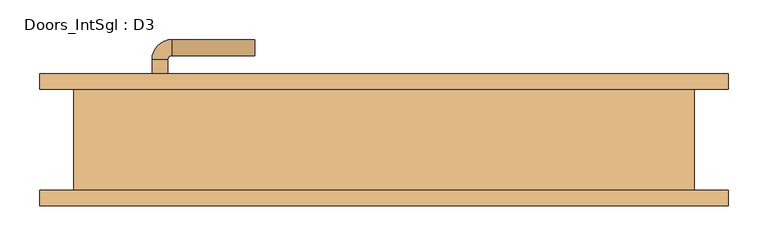
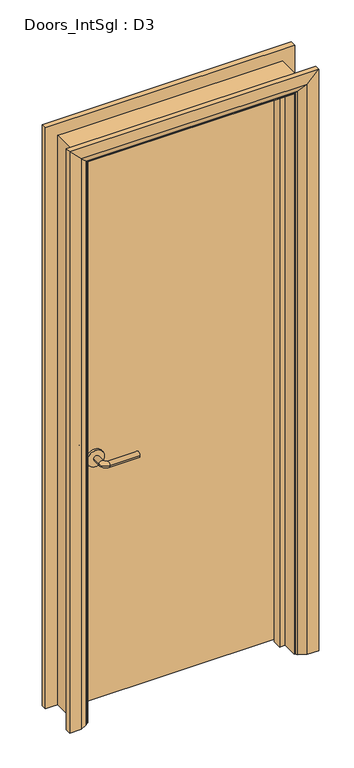
"""IFC4 building model written with IfcOpenShell, lengths in millimetres: door geometry, Doors_IntSgl : D3."""

from ifc_helpers import new_model, si_unit, point, frame, frame_2d, origin, place, context, project, spatial, polyline, circle_curve, ellipse_curve, trimmed, segment, composite_curve, outline, extrude, faceted_brep, source, transform, mapped, element, save
from ifc_brep_helpers import plane_surface, cylinder_surface, revolved_surface, advanced_brep


def doors_intsgl_d3_a25f8c6e(model_context):
    return source(origin(), model_context, "Body", "SolidModel", [
        advanced_brep(
        [(-293.05, 17.5, 900.0), (-273.05, 17.5, 900.0), (-273.05, -12.5, 900.0), (-293.05, -12.5, 900.0), (-268.05, -17.5, 900.0), (-268.05, -37.5, 900.0), (-163.05, -37.5, 900.0), (-163.05, -17.5, 900.0)],
        [
            (0, 1, circle_curve(frame((-283.05, 17.5, 900.0), z_axis=(0.0, 1.0, 0.0), x_axis=(1.0, 0.0, 0.0)), 10.0)),
            (1, 0, circle_curve(frame((-283.05, 17.5, 900.0), z_axis=(0.0, 1.0, 0.0), x_axis=(1.0, 0.0, 0.0)), 10.0)),
            (1, 2),
            (2, 3, circle_curve(frame((-283.05, -12.5, 900.0), z_axis=(0.0, 1.0, 0.0), x_axis=(1.0, 0.0, 0.0)), 10.0)),
            (3, 0),
            (3, 2, circle_curve(frame((-283.05, -12.5, 900.0), z_axis=(0.0, 1.0, 0.0), x_axis=(1.0, 0.0, 0.0)), 10.0)),
            (4, 5, circle_curve(frame((-268.05, -27.5, 900.0), z_axis=(-1.0, 0.0, 0.0), x_axis=(0.0, 1.0, 0.0)), 10.0)),
            (5, 3, circle_curve(frame((-268.05, -12.5, 900.0), z_axis=(0.0, 0.0, -1.0), x_axis=(-1.0, 0.0, 0.0)), 25.0)),
            (2, 4, circle_curve(frame((-268.05, -12.5, 900.0), z_axis=(0.0, 0.0, 1.0), x_axis=(-1.0, 0.0, 0.0)), 5.0)),
            (5, 4, circle_curve(frame((-268.05, -27.5, 900.0), z_axis=(-1.0, 0.0, 0.0), x_axis=(0.0, 1.0, 0.0)), 10.0)),
            (6, 7, circle_curve(frame((-163.05, -27.5, 900.0), z_axis=(1.0, 0.0, 0.0), x_axis=(0.0, 1.0, 0.0)), 10.0)),
            (7, 6, circle_curve(frame((-163.05, -27.5, 900.0), z_axis=(1.0, 0.0, 0.0), x_axis=(0.0, 1.0, 0.0)), 10.0)),
            (4, 7),
            (6, 5),
        ],
        [
            plane_surface(frame((-283.05, 17.5, 900.0), z_axis=(0.0, 1.0, 0.0), x_axis=(0.0, 0.0, 1.0))),
            cylinder_surface(frame((-283.05, 17.5, 900.0), z_axis=(0.0, 1.0, 0.0), x_axis=(1.0, 0.0, 0.0)), 10.0),
            revolved_surface(trimmed(ellipse_curve(frame((-283.05, -12.5, 900.0), z_axis=(0.0, -1.0, 0.0), x_axis=(1.0, 0.0, 0.0)), 10.0, 10.0), [point((-293.05, -12.5, 900.0))], [point((-273.05, -12.5, 900.0))], True, "CARTESIAN"), (-268.05, -12.5, 900.0), (0.0, 0.0, -1.0)),
            revolved_surface(trimmed(ellipse_curve(frame((-283.05, -12.5, 900.0), z_axis=(0.0, -1.0, 0.0), x_axis=(1.0, 0.0, 0.0)), 10.0, 10.0), [point((-273.05, -12.5, 900.0))], [point((-293.05, -12.5, 900.0))], True, "CARTESIAN"), (-268.05, -12.5, 900.0), (0.0, 0.0, -1.0)),
            plane_surface(frame((-163.05, -27.5, 900.0), z_axis=(1.0, 0.0, 0.0), x_axis=(0.0, 0.0, 1.0))),
            cylinder_surface(frame((-268.05, -27.5, 900.0), z_axis=(-1.0, 0.0, 0.0), x_axis=(0.0, 1.0, 0.0)), 10.0),
        ],
        [
            (0, [[1, 2]]),
            (1, [[3, 4, 5, -2]]),
            (1, [[-5, 6, -3, -1]]),
            (2, [[7, 8, -4, 9]]),
            (3, [[10, -9, -6, -8]]),
            (4, [[11, 12]]),
            (5, [[13, -11, 14, -7]]),
            (5, [[-14, -12, -13, -10]]),
        ],
    ),
        extrude(outline(composite_curve([segment(trimmed(circle_curve(frame_2d((900.0, -285.55)), 30.0), [point((900.0, -315.55))], [point((900.0, -255.55))], False, "CARTESIAN"), True, "CONTINUOUS"), segment(trimmed(circle_curve(frame_2d((900.0, -285.55)), 30.0), [point((900.0, -255.55))], [point((900.0, -315.55))], False, "CARTESIAN"), True, "CONTINUOUS")], self_intersect=False)), frame((0.0, 17.5, 0.0), z_axis=(0.0, 1.0, 0.0), x_axis=(0.0, 0.0, 1.0)), (0.0, 0.0, 1.0), 8.0),
        advanced_brep(
        [(-293.05, 71.5, 900.0), (-273.05, 71.5, 900.0), (-293.05, 101.5, 900.0), (-273.05, 101.5, 900.0), (-268.05, 106.5, 900.0), (-268.05, 126.5, 900.0), (-163.05, 126.5, 900.0), (-163.05, 106.5, 900.0)],
        [
            (0, 1, circle_curve(frame((-283.05, 71.5, 900.0), z_axis=(0.0, -1.0, 0.0), x_axis=(1.0, 0.0, 0.0)), 10.0)),
            (1, 0, circle_curve(frame((-283.05, 71.5, 900.0), z_axis=(0.0, -1.0, 0.0), x_axis=(1.0, 0.0, 0.0)), 10.0)),
            (0, 2),
            (2, 3, circle_curve(frame((-283.05, 101.5, 900.0), z_axis=(0.0, -1.0, 0.0), x_axis=(1.0, 0.0, 0.0)), 10.0)),
            (3, 1),
            (3, 2, circle_curve(frame((-283.05, 101.5, 900.0), z_axis=(0.0, -1.0, 0.0), x_axis=(1.0, 0.0, 0.0)), 10.0)),
            (4, 3, circle_curve(frame((-268.05, 101.5, 900.0), z_axis=(0.0, 0.0, 1.0), x_axis=(-1.0, 0.0, 0.0)), 5.0)),
            (2, 5, circle_curve(frame((-268.05, 101.5, 900.0), z_axis=(0.0, 0.0, -1.0), x_axis=(-1.0, 0.0, 0.0)), 25.0)),
            (5, 4, circle_curve(frame((-268.05, 116.5, 900.0), z_axis=(-1.0, 0.0, 0.0), x_axis=(0.0, -1.0, 0.0)), 10.0)),
            (4, 5, circle_curve(frame((-268.05, 116.5, 900.0), z_axis=(-1.0, 0.0, 0.0), x_axis=(0.0, -1.0, 0.0)), 10.0)),
            (6, 7, circle_curve(frame((-163.05, 116.5, 900.0), z_axis=(1.0, 0.0, 0.0), x_axis=(0.0, -1.0, 0.0)), 10.0)),
            (7, 6, circle_curve(frame((-163.05, 116.5, 900.0), z_axis=(1.0, 0.0, 0.0), x_axis=(0.0, -1.0, 0.0)), 10.0)),
            (5, 6),
            (7, 4),
        ],
        [
            plane_surface(frame((-283.05, 71.5, 900.0), z_axis=(0.0, -1.0, 0.0), x_axis=(0.0, 0.0, 1.0))),
            cylinder_surface(frame((-283.05, 71.5, 900.0), z_axis=(0.0, -1.0, 0.0), x_axis=(1.0, 0.0, 0.0)), 10.0),
            revolved_surface(trimmed(ellipse_curve(frame((-283.05, 101.5, 900.0), z_axis=(0.0, -1.0, 0.0), x_axis=(1.0, 0.0, 0.0)), 10.0, 10.0), [point((-293.05, 101.5, 900.0))], [point((-273.05, 101.5, 900.0))], True, "CARTESIAN"), (-268.05, 101.5, 900.0), (0.0, 0.0, -1.0)),
            revolved_surface(trimmed(ellipse_curve(frame((-283.05, 101.5, 900.0), z_axis=(0.0, -1.0, 0.0), x_axis=(1.0, 0.0, 0.0)), 10.0, 10.0), [point((-273.05, 101.5, 900.0))], [point((-293.05, 101.5, 900.0))], True, "CARTESIAN"), (-268.05, 101.5, 900.0), (0.0, 0.0, -1.0)),
            plane_surface(frame((-163.05, 116.5, 900.0), z_axis=(1.0, 0.0, 0.0), x_axis=(0.0, 0.0, 1.0))),
            cylinder_surface(frame((-268.05, 116.5, 900.0), z_axis=(-1.0, 0.0, 0.0), x_axis=(0.0, -1.0, 0.0)), 10.0),
        ],
        [
            (0, [[1, 2]]),
            (1, [[-1, 3, 4, 5]]),
            (1, [[-2, -5, 6, -3]]),
            (2, [[7, -4, 8, 9]]),
            (3, [[-8, -6, -7, 10]]),
            (4, [[11, 12]]),
            (5, [[-9, 13, -12, 14]]),
            (5, [[-10, -14, -11, -13]]),
        ],
    ),
        extrude(outline(composite_curve([segment(trimmed(circle_curve(frame_2d((900.0, -285.55)), 30.0), [point((900.0, -315.55))], [point((900.0, -255.55))], False, "CARTESIAN"), True, "CONTINUOUS"), segment(trimmed(circle_curve(frame_2d((900.0, -285.55)), 30.0), [point((900.0, -255.55))], [point((900.0, -315.55))], False, "CARTESIAN"), True, "CONTINUOUS")], self_intersect=False)), frame((0.0, 63.5, 0.0), z_axis=(0.0, 1.0, 0.0), x_axis=(0.0, 0.0, 1.0)), (0.0, 0.0, 1.0), 8.0),
        extrude(outline(polyline([(358.05, 25.5), (-358.05, 25.5), (-358.05, 63.5), (358.05, 63.5), (358.05, 25.5)])), frame((0.0, 0.0, 8.0), z_axis=(0.0, 0.0, 1.0), x_axis=(1.0, 0.0, 0.0)), (0.0, 0.0, 1.0), 2060.0),
        advanced_brep(
        [(435.05, 83.5, 0.0), (435.05, 63.5, 0.0), (365.05, 63.5, 0.0), (369.05, 69.5, 0.0), (395.05, 83.5, 0.0), (435.05, 83.5, 2145.0), (435.05, 63.5, 2145.0), (-435.05, 63.5, 2145.0), (-435.05, 63.5, 0.0), (-365.05, 63.5, 0.0), (-365.05, 63.5, 2075.0), (365.05, 63.5, 2075.0), (369.05, 69.5, 2079.0), (395.05, 83.5, 2105.0), (-395.05, 83.5, 2105.0), (-395.05, 83.5, 0.0), (-435.05, 83.5, 0.0), (-435.05, 83.5, 2145.0), (-369.05, 69.5, 0.0), (-369.05, 69.5, 2079.0)],
        [
            (0, 1),
            (1, 2),
            (2, 3, circle_curve(frame((373.05, 62.5, 0.0), z_axis=(0.0, 0.0, -1.0), x_axis=(1.0, 0.0, 0.0)), 8.0622577)),
            (3, 4),
            (4, 0),
            (0, 5),
            (5, 6),
            (6, 1),
            (6, 7),
            (7, 8),
            (8, 9),
            (9, 10),
            (10, 11),
            (11, 2),
            (11, 12, ellipse_curve(frame((373.05, 62.5, 2083.0), z_axis=(0.7071067811865475, 0.0, -0.7071067811865475), x_axis=(-0.7071067811865474, 0.0, -0.7071067811865476)), 11.4017543, 8.0622577)),
            (12, 3),
            (12, 13),
            (13, 4),
            (13, 14),
            (14, 15),
            (15, 16),
            (16, 17),
            (17, 5),
            (7, 17),
            (16, 8),
            (15, 18),
            (18, 9, circle_curve(frame((-373.05, 62.5, 0.0), z_axis=(0.0, 0.0, -1.0), x_axis=(-1.0, 0.0, 0.0)), 8.0622577)),
            (19, 10, ellipse_curve(frame((-373.05, 62.5, 2083.0), z_axis=(-0.7071067811865475, 0.0, -0.7071067811865475), x_axis=(-0.7071067811865474, 0.0, 0.7071067811865476)), 11.4017543, 8.0622577)),
            (18, 19),
            (14, 19),
            (19, 12),
        ],
        [
            plane_surface(frame((365.05, 63.5, 0.0), z_axis=(0.0, 0.0, -1.0), x_axis=(0.0, -1.0, 0.0))),
            plane_surface(frame((435.05, 83.5, 0.0), z_axis=(1.0, 0.0, 0.0), x_axis=(0.0, 0.0, 1.0))),
            plane_surface(frame((435.05, 63.5, 0.0), z_axis=(0.0, -1.0, 0.0), x_axis=(0.0, 0.0, 1.0))),
            cylinder_surface(frame((373.05, 62.5, 0.0), z_axis=(0.0, 0.0, -1.0), x_axis=(1.0, 0.0, 0.0)), 8.0622577),
            plane_surface(frame((369.05, 69.5, 0.0), z_axis=(-0.4740998230350126, 0.880471099922178, 0.0), x_axis=(0.0, 0.0, 1.0))),
            plane_surface(frame((395.05, 83.5, 0.0), z_axis=(0.0, 1.0, 0.0), x_axis=(0.0, 0.0, 1.0))),
            plane_surface(frame((-435.05, 83.5, 2145.0), z_axis=(-1.0, 0.0, 0.0), x_axis=(0.0, 0.0, -1.0))),
            plane_surface(frame((-365.05, 63.5, 0.0), z_axis=(0.0, 0.0, -1.0), x_axis=(0.0, -1.0, 0.0))),
            cylinder_surface(frame((-373.05, 62.5, 2075.0), z_axis=(0.0, 0.0, 1.0), x_axis=(-1.0, 0.0, 0.0)), 8.0622577),
            plane_surface(frame((-369.05, 69.5, 2079.0), z_axis=(0.47409982303501824, 0.8804710999221749, 0.0), x_axis=(0.0, 0.0, -1.0))),
            plane_surface(frame((435.05, 83.5, 2145.0), z_axis=(0.0, 0.0, 1.0), x_axis=(-1.0, 0.0, 0.0))),
            cylinder_surface(frame((365.05, 62.5, 2083.0), z_axis=(1.0, 0.0, 0.0), x_axis=(0.0, 0.0, 1.0)), 8.0622577),
            plane_surface(frame((369.05, 69.5, 2079.0), z_axis=(0.0, 0.8804710999221764, -0.4740998230350154), x_axis=(-1.0, 0.0, 0.0))),
        ],
        [
            (0, [[1, 2, 3, 4, 5]]),
            (1, [[-1, 6, 7, 8]]),
            (2, [[-2, -8, 9, 10, 11, 12, 13, 14]]),
            (3, [[-3, -14, 15, 16]]),
            (4, [[-4, -16, 17, 18]]),
            (5, [[-5, -18, 19, 20, 21, 22, 23, -6]]),
            (6, [[24, -22, 25, -10]]),
            (7, [[-21, 26, 27, -11, -25]]),
            (8, [[28, -12, -27, 29]]),
            (9, [[30, -29, -26, -20]]),
            (10, [[-7, -23, -24, -9]]),
            (11, [[-15, -13, -28, 31]]),
            (12, [[-17, -31, -30, -19]]),
        ],
    ),
        extrude(outline(polyline([(0.0, -360.05), (0.0, -341.05), (2051.0, -341.05), (2051.0, 341.05), (0.0, 341.05), (0.0, 360.05), (2070.0, 360.05), (2070.0, -360.05), (0.0, -360.05)])), frame((0.0, -8.5, 0.0), z_axis=(0.0, 1.0, 0.0), x_axis=(0.0, 0.0, 1.0)), (0.0, 0.0, 1.0), 32.0),
        advanced_brep(
        [(-435.05, -83.5, 0.0), (-435.05, -63.5, 0.0), (-365.05, -63.5, 0.0), (-369.05, -69.5, 0.0), (-395.05, -83.5, 0.0), (-435.05, -83.5, 2145.0), (-435.05, -63.5, 2145.0), (-365.05, -63.5, 2075.0), (-369.05, -69.5, 2079.0), (-395.05, -83.5, 2105.0), (435.05, -83.5, 0.0), (395.05, -83.5, 0.0), (369.05, -69.5, 0.0), (365.05, -63.5, 0.0), (435.05, -63.5, 0.0), (435.05, -83.5, 2145.0), (395.05, -83.5, 2105.0), (369.05, -69.5, 2079.0), (365.05, -63.5, 2075.0), (435.05, -63.5, 2145.0)],
        [
            (0, 1),
            (1, 2),
            (2, 3, circle_curve(frame((-373.05, -62.5, 0.0), z_axis=(0.0, 0.0, -1.0), x_axis=(-1.0, 0.0, 0.0)), 8.0622577)),
            (3, 4),
            (4, 0),
            (0, 5),
            (5, 6),
            (6, 1),
            (6, 7),
            (7, 2),
            (7, 8, ellipse_curve(frame((-373.05, -62.5, 2083.0), z_axis=(-0.7071067811865475, 0.0, -0.7071067811865475), x_axis=(0.7071067811865474, 0.0, -0.7071067811865476)), 11.4017543, 8.0622577)),
            (8, 3),
            (8, 9),
            (9, 4),
            (9, 5),
            (10, 11),
            (11, 12),
            (12, 13, circle_curve(frame((373.05, -62.5, 0.0), z_axis=(0.0, 0.0, -1.0), x_axis=(1.0, 0.0, 0.0)), 8.0622577)),
            (13, 14),
            (14, 10),
            (15, 16),
            (16, 11),
            (10, 15),
            (16, 17),
            (17, 12),
            (17, 18, ellipse_curve(frame((373.05, -62.5, 2083.0), z_axis=(0.7071067811865475, 0.0, -0.7071067811865475), x_axis=(0.7071067811865474, 0.0, 0.7071067811865476)), 11.4017543, 8.0622577)),
            (18, 13),
            (18, 19),
            (19, 14),
            (19, 15),
            (5, 15),
            (19, 6),
            (18, 7),
            (17, 8),
            (16, 9),
        ],
        [
            plane_surface(frame((-365.05, -136.3010989, 0.0), z_axis=(0.0, 0.0, -1.0), x_axis=(1.0, 0.0, 0.0))),
            plane_surface(frame((-435.05, -83.5, 0.0), z_axis=(-1.0, 0.0, 0.0), x_axis=(0.0, 0.0, 1.0))),
            plane_surface(frame((-435.05, -63.5, 0.0), z_axis=(0.0, 1.0, 0.0), x_axis=(0.0, 0.0, 1.0))),
            cylinder_surface(frame((-373.05, -62.5, 0.0), z_axis=(0.0, 0.0, -1.0), x_axis=(-1.0, 0.0, 0.0)), 8.0622577),
            plane_surface(frame((-369.05, -69.5, 0.0), z_axis=(0.4740998230350183, -0.8804710999221749, 0.0), x_axis=(0.0, 0.0, 1.0))),
            plane_surface(frame((-395.05, -83.5, 0.0), z_axis=(0.0, -1.0, 0.0), x_axis=(0.0, 0.0, 1.0))),
            plane_surface(frame((365.05, -136.3010989, 0.0), z_axis=(0.0, 0.0, -1.0), x_axis=(-1.0, 0.0, 0.0))),
            plane_surface(frame((395.05, -83.5, 2105.0), z_axis=(0.0, -1.0, 0.0), x_axis=(0.0, 0.0, -1.0))),
            plane_surface(frame((369.05, -69.5, 2079.0), z_axis=(-0.4740998230350183, -0.8804710999221749, 0.0), x_axis=(0.0, 0.0, -1.0))),
            cylinder_surface(frame((373.05, -62.5, 2075.0), z_axis=(0.0, 0.0, 1.0), x_axis=(1.0, 0.0, 0.0)), 8.0622577),
            plane_surface(frame((435.05, -63.5, 2145.0), z_axis=(0.0, 1.0, 0.0), x_axis=(0.0, 0.0, -1.0))),
            plane_surface(frame((435.05, -83.5, 2145.0), z_axis=(1.0, 0.0, 0.0), x_axis=(0.0, 0.0, -1.0))),
            plane_surface(frame((-435.05, -83.5, 2145.0), z_axis=(0.0, 0.0, 1.0), x_axis=(1.0, 0.0, 0.0))),
            plane_surface(frame((-435.05, -63.5, 2145.0), z_axis=(0.0, 1.0, 0.0), x_axis=(1.0, 0.0, 0.0))),
            cylinder_surface(frame((-365.05, -62.5, 2083.0), z_axis=(-1.0, 0.0, 0.0), x_axis=(0.0, 0.0, 1.0)), 8.0622577),
            plane_surface(frame((-369.05, -69.5, 2079.0), z_axis=(0.0, -0.8804710999221749, -0.4740998230350183), x_axis=(1.0, 0.0, 0.0))),
            plane_surface(frame((-395.05, -83.5, 2105.0), z_axis=(0.0, -1.0, 0.0), x_axis=(1.0, 0.0, 0.0))),
        ],
        [
            (0, [[1, 2, 3, 4, 5]]),
            (1, [[-1, 6, 7, 8]]),
            (2, [[-2, -8, 9, 10]]),
            (3, [[-3, -10, 11, 12]]),
            (4, [[-4, -12, 13, 14]]),
            (5, [[-5, -14, 15, -6]]),
            (6, [[16, 17, 18, 19, 20]]),
            (7, [[21, 22, -16, 23]]),
            (8, [[24, 25, -17, -22]]),
            (9, [[26, 27, -18, -25]]),
            (10, [[28, 29, -19, -27]]),
            (11, [[30, -23, -20, -29]]),
            (12, [[-7, 31, -30, 32]]),
            (13, [[-9, -32, -28, 33]]),
            (14, [[-11, -33, -26, 34]]),
            (15, [[-13, -34, -24, 35]]),
            (16, [[-15, -35, -21, -31]]),
        ],
    ),
        faceted_brep([(-360.05, 63.5, 0.0), (-360.05, -63.5, 0.0), (-392.05, -63.5, 0.0), (-392.05, 63.5, 0.0), (-360.05, 63.5, 2070.0), (-360.05, -63.5, 2070.0), (-392.05, -63.5, 2102.0), (-392.05, 63.5, 2102.0), (360.05, 63.5, 0.0), (392.05, 63.5, 0.0), (392.05, -63.5, 0.0), (360.05, -63.5, 0.0), (360.05, 63.5, 2070.0), (392.05, 63.5, 2102.0), (392.05, -63.5, 2102.0), (360.05, -63.5, 2070.0)], [[[0, 1, 2, 3]], [[1, 0, 4, 5]], [[2, 1, 5, 6]], [[3, 2, 6, 7]], [[0, 3, 7, 4]], [[8, 9, 10, 11]], [[12, 13, 9, 8]], [[13, 14, 10, 9]], [[14, 15, 11, 10]], [[15, 12, 8, 11]], [[5, 4, 12, 15]], [[6, 5, 15, 14]], [[7, 6, 14, 13]], [[4, 7, 13, 12]]]),
    ])


if __name__ == "__main__":
    model = new_model("IFC4")
    model_context = context("Model", 3, world=origin())
    ifc_project = project(units=[si_unit("LENGTHUNIT", "METRE", prefix="MILLI")], contexts=[model_context])
    site = spatial("IfcSite", under=ifc_project)
    building = spatial("IfcBuilding", under=site)
    placement = place(None, origin())
    doors_intsgl_d3_shape = doors_intsgl_d3_a25f8c6e(model_context)
    element("IfcDoor", 1, ObjectType="Doors_IntSgl : D3", at=placement, inside=building, context=model_context, shape_type="MappedRepresentation", body=[
        mapped(doors_intsgl_d3_shape, transform((0.0, 0.0, 0.0), x_axis=(1.0, 0.0, 0.0), y_axis=(0.0, 1.0, 0.0), z_axis=(0.0, 0.0, 1.0))),
    ])
    save(model, "model.ifc")

# Revit data of these elements
# Type "Doors_IntSgl : D3"
#   Type Mark = "49"
#   Type Comments = "Internal Single"
#   Operation = "SingleSwingRight"
#   Manufacturer = "Revit"
#   Keynote = "L20"
#   Description = "Internal Single Door"
#   Analytic Construction = "Metal"
#   UnderCut = 0' - 0.31496"
#   Tolerance = 0' - 0.07874"
#   Thickness = 0' - 1.49606"
#   Thermal Resistance (R) = 0.270117 (m²·K)/W
#   Structural Tolerance = 0' - 0.31496"
#   StopDepth = 0' - 1.25984"
#   Stop Thickness = 0' - 0.74803"
#   Rough Width = 2' - 7 1/2"
#   Rough Height = 6' - 11.07087"
#   Height to Top Lock Rail = 3' - 3.37008"
#   Heat Transfer Coefficient (U) = 3.7021 W/(m²·K)
#   Handle Z Distance = 2' - 11.43307"
#   Handle X Distance = 0' - 2.95276"
#   Frame Thickness = 0' - 1.25984"
#   Door Panel Width = 2' - 4.19291"
#   Door Panel Thickness = 0' - 1.49606"
#   Door Panel Offset = 0' - 0"
#   Height = 6' - 11.07087"
#   Width = 2' - 7 1/2"
#   Door Panel Height = 6' - 9.10236"
#   Architrave Setback = 0' - 0.19685"
#   Vis - Ironmongery = yes
#   Material Ironmongery = Door - Handle
#   Material Frame = Door - Frame/Mullion (1)
#   Material Door = Door - Panel
#   Material Architrave = Door - Architrave
#   Visual Light Transmittance = 0
#   Solar Heat Gain Coefficient = 0
#   Function = (empty or 0)
#   Wall Closure = (empty or 0)
# Element 1 (IfcDoor, "Doors_IntSgl : D3")
#   Materials on its faces: "Door - Architrave", "Door - Handle", "Door - Frame/Mullion (1)", "Door - Panel"
# Materials
#   "Door - Handle": colour RGB 0 0 0, transparency 0, Keynote = "P21", Cost = 0
#   "Door - Frame/Mullion (1)": class "Wood", colour RGB 212 179 113, transparency 0, Keynote = "L20", Cost = 0
#   "Door - Panel": class "Wood", colour RGB 210 159 95, transparency 0, Keynote = "L20", Cost = 0
#   "Door - Architrave": class "Wood", colour RGB 154 90 5, transparency 0, Keynote = "P20", Cost = 0
